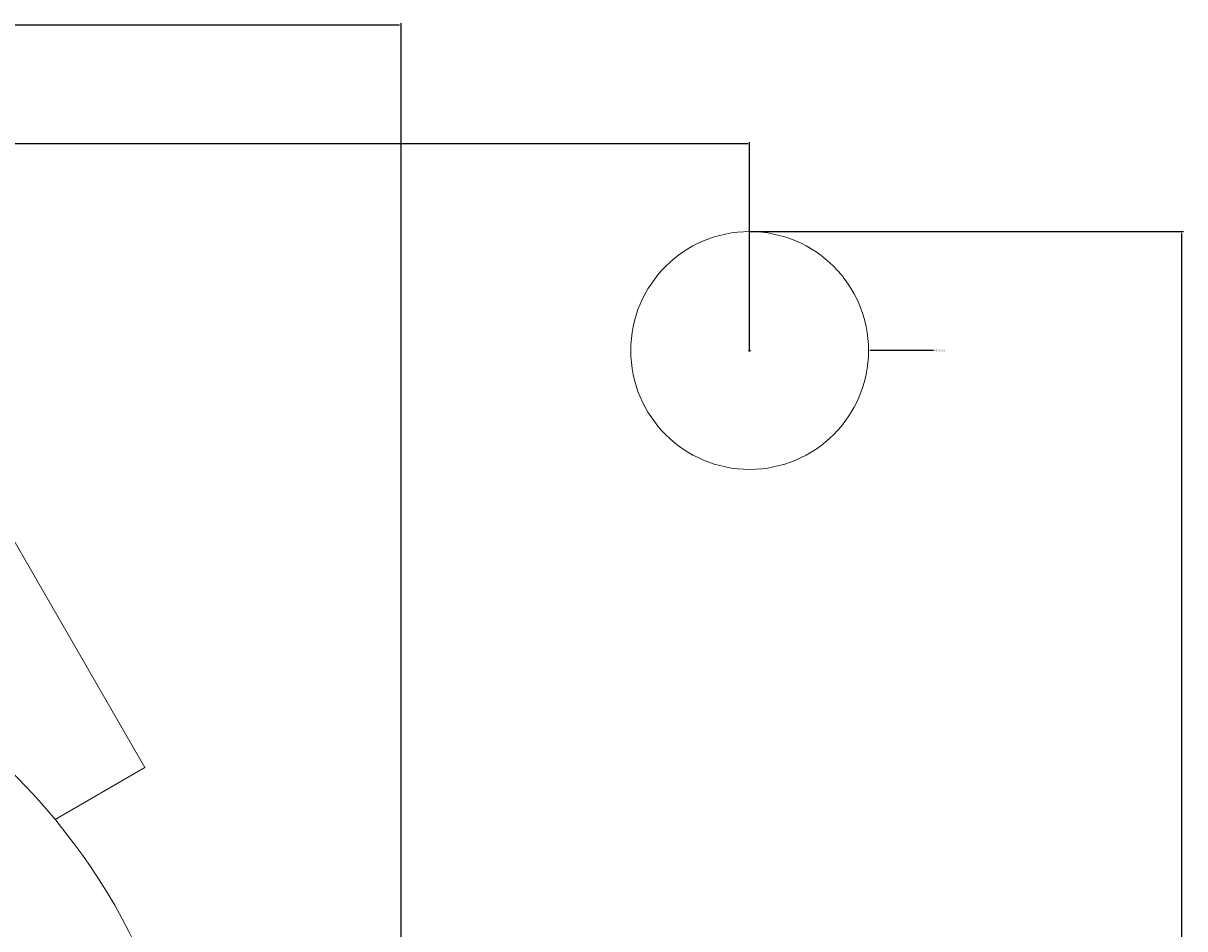
# Model space of a CAD drawing. Units: inches. Extents: x 1095 to 1408, y -20 to 240.
# Tile 8 of 8: x 1294 to 1408, y 152 to 240. Entities that reach past the tile are written whole.
import ezdxf

# ---------------------------------------------------------------- set-up
doc = ezdxf.new("R2010")
doc.units = ezdxf.units.IN
doc.header["$MEASUREMENT"] = 0
doc.layers.add('M-CONS', color=8, linetype='Continuous', lineweight=18)
doc.layers.add('M-DIMS', color=2, linetype='Continuous', lineweight=18)
doc.styles.get("Standard").update_dxf_attribs({"font": 'arial.ttf'})
doc.dimstyles.get("Standard").update_dxf_attribs({"dimtxt": 0.18, "dimasz": 0.18, "dimexe": 0.18, "dimexo": 0.0625, "dimgap": 0.09, "dimtad": 0, "dimtih": 1, "dimtoh": 1, "dimdec": 4, "dimzin": 0, "dimdsep": 46, "dimtxsty": 'Standard', "dimcen": 0.09, "dimadec": 0, "dimazin": 0, "dimtfac": 1, "dimtdec": 4, "dimtofl": 0, "dimtmove": 0, "dimatfit": 3, "dimfxl": 1, "dimtolj": 1, "dimtzin": 0, "dimarcsym": 0})

# ---------------------------------------------------------------- blocks, each defined once
blk = doc.blocks.new('*D2')
at = {"layer": 'Defpoints', "color": 0, "transparency": 16777216}
for p in [(1365.18, 219.6), (1407.33, 219.6), (1387.18, 0)]:
    blk.add_point(p, dxfattribs=at)
at = {"layer": 'M-DIMS', "color": 0, "lineweight": -2, "transparency": 16777216}
for p, q in [((1365.25, 219.6), (1407.51, 219.6)), ((1407.33, 219.42), (1407.33, 109.98)), ((1407.33, 0.18), (1407.33, 109.62)), ((1387.25, 0), (1407.51, 0))]:
    blk.add_line(p, q, dxfattribs=at)
at = {"layer": 'M-DIMS', "color": 0, "transparency": 16777216}
for points in [[(1407.3, 219.42), (1407.36, 219.42), (1407.33, 219.6)], [(1407.3, 0.18), (1407.36, 0.18), (1407.33, 0)]]:
    blk.add_solid(points, dxfattribs=at)
at = {"layer": 'M-DIMS', "color": 0, "transparency": 16777216, "insert": (1407.33, 109.8), "char_height": 0.18, "attachment_point": 5}
blk.add_mtext('\\A1;219.6', dxfattribs=at)
blk = doc.blocks.new('*D5')
at = {"layer": 'Defpoints', "color": 0, "transparency": 16777216}
for p in [(1365.18, 228.15), (1137.18, 208), (1365.18, 208)]:
    blk.add_point(p, dxfattribs=at)
at = {"layer": 'M-DIMS', "color": 0, "lineweight": -2, "transparency": 16777216}
for p, q in [((1137.18, 208.06), (1137.18, 228.33)), ((1137.36, 228.15), (1250.89, 228.15)), ((1365, 228.15), (1251.47, 228.15)), ((1365.18, 208.06), (1365.18, 228.33))]:
    blk.add_line(p, q, dxfattribs=at)
at = {"layer": 'M-DIMS', "color": 0, "transparency": 16777216}
for points in [[(1137.36, 228.18), (1137.36, 228.12), (1137.18, 228.15)], [(1365, 228.18), (1365, 228.12), (1365.18, 228.15)]]:
    blk.add_solid(points, dxfattribs=at)
at = {"layer": 'M-DIMS', "color": 0, "transparency": 16777216, "insert": (1251.18, 228.15), "char_height": 0.18, "attachment_point": 5}
blk.add_mtext('\\A1;228', dxfattribs=at)
blk = doc.blocks.new('*D9')
at = {"layer": 'Defpoints', "color": 0, "transparency": 16777216}
for p in [(1331.18, 239.75), (1171.18, 124), (1331.18, 124)]:
    blk.add_point(p, dxfattribs=at)
at = {"layer": 'M-DIMS', "color": 0, "lineweight": -2, "transparency": 16777216}
for p, q in [((1171.18, 124.06), (1171.18, 239.93)), ((1171.36, 239.75), (1250.9, 239.75)), ((1331, 239.75), (1251.46, 239.75)), ((1331.18, 124.06), (1331.18, 239.93))]:
    blk.add_line(p, q, dxfattribs=at)
at = {"layer": 'M-DIMS', "color": 0, "transparency": 16777216}
for points in [[(1171.36, 239.78), (1171.36, 239.72), (1171.18, 239.75)], [(1331, 239.78), (1331, 239.72), (1331.18, 239.75)]]:
    blk.add_solid(points, dxfattribs=at)
at = {"layer": 'M-DIMS', "color": 0, "transparency": 16777216, "insert": (1251.18, 239.75), "char_height": 0.18, "attachment_point": 5}
blk.add_mtext('\\A1;160', dxfattribs=at)
blk = doc.blocks.new('*D17')
at = {"layer": 'Defpoints', "color": 0, "transparency": 16777216}
for p in [(1353.58, 208), (1376.78, 208)]:
    blk.add_point(p, dxfattribs=at)
at = {"layer": 'M-DIMS', "color": 0, "lineweight": -2, "transparency": 16777216}
for p, q in [((1365.09, 208), (1365.27, 208)), ((1365.18, 207.91), (1365.18, 208.09)), ((1383.13, 208), (1376.96, 208))]:
    blk.add_line(p, q, dxfattribs=at)
at = {"layer": 'M-DIMS', "color": 0, "transparency": 16777216}
blk.add_solid([(1376.96, 208.03), (1376.96, 207.97), (1376.78, 208)], dxfattribs=at)
at = {"layer": 'M-DIMS', "color": 0, "transparency": 16777216, "insert": (1383.74, 208), "char_height": 0.18, "attachment_point": 5}
blk.add_mtext('\\A1;4X ∅23.2', dxfattribs=at)

msp = doc.modelspace()

# ---------------------------------------------------------------- linework, layer by layer
at = {"layer": 'M-CONS', "elevation": 377.783}
msp.add_lwpolyline([(1297.418, 162.241), (1306.184, 167.301), (1291.184, 193.282), (1211.184, 193.282), (1196.184, 167.301), (1204.949, 162.241)], dxfattribs=at)
at = {"layer": 'M-CONS'}
for centre, radius in [((1365.184, 208, 397.783), 11.6), ((1251.184, 124, 377.783), 60)]:
    msp.add_circle(centre, radius, dxfattribs=at)

# ---------------------------------------------------------------- dimensions: what is measured, and where the dimension line sits
at = {"layer": 'M-DIMS'}
for base, p1, p2, picture, middle in [((1331.184, 239.75), (1171.184, 124), (1331.184, 124), '*D9', (1251.184, 239.75)), ((1365.184, 228.15), (1137.184, 208), (1365.184, 208), '*D5', (1251.184, 228.15))]:
    dim = msp.add_linear_dim(base=base, p1=p1, p2=p2, dimstyle='Standard', override={"dimdec": 0, "dimlfac": 1, "dimrnd": 0, "dimzin": 0, "dimdsep": 46, "dimlunit": 2}, dxfattribs=at)
    dim.commit()
    dim.dimension.update_dxf_attribs({"geometry": picture, "text_midpoint": middle})
dim = msp.add_linear_dim(base=(1407.334, 219.6), p1=(1387.184, 0), p2=(1365.184, 219.6), angle=90, dimstyle='Standard', override={"dimdec": 1, "dimlfac": 1, "dimrnd": 0, "dimzin": 0, "dimdsep": 46, "dimlunit": 2}, dxfattribs=at)
dim.commit()
dim.dimension.update_dxf_attribs({"geometry": '*D2', "text_midpoint": (1407.334, 109.8)})
dim = msp.add_diameter_dim_2p(p1=(1353.584, 208), p2=(1376.784, 208), text='4X <>', dimstyle='Standard', override={"dimdec": 1, "dimlfac": 1, "dimrnd": 0, "dimzin": 0, "dimdsep": 46, "dimlunit": 2}, dxfattribs=at)
dim.commit()
dim.dimension.update_dxf_attribs({"geometry": '*D17', "text_midpoint": (1383.744, 208), "dimtype": 163})

doc.saveas('drawing.dxf')
